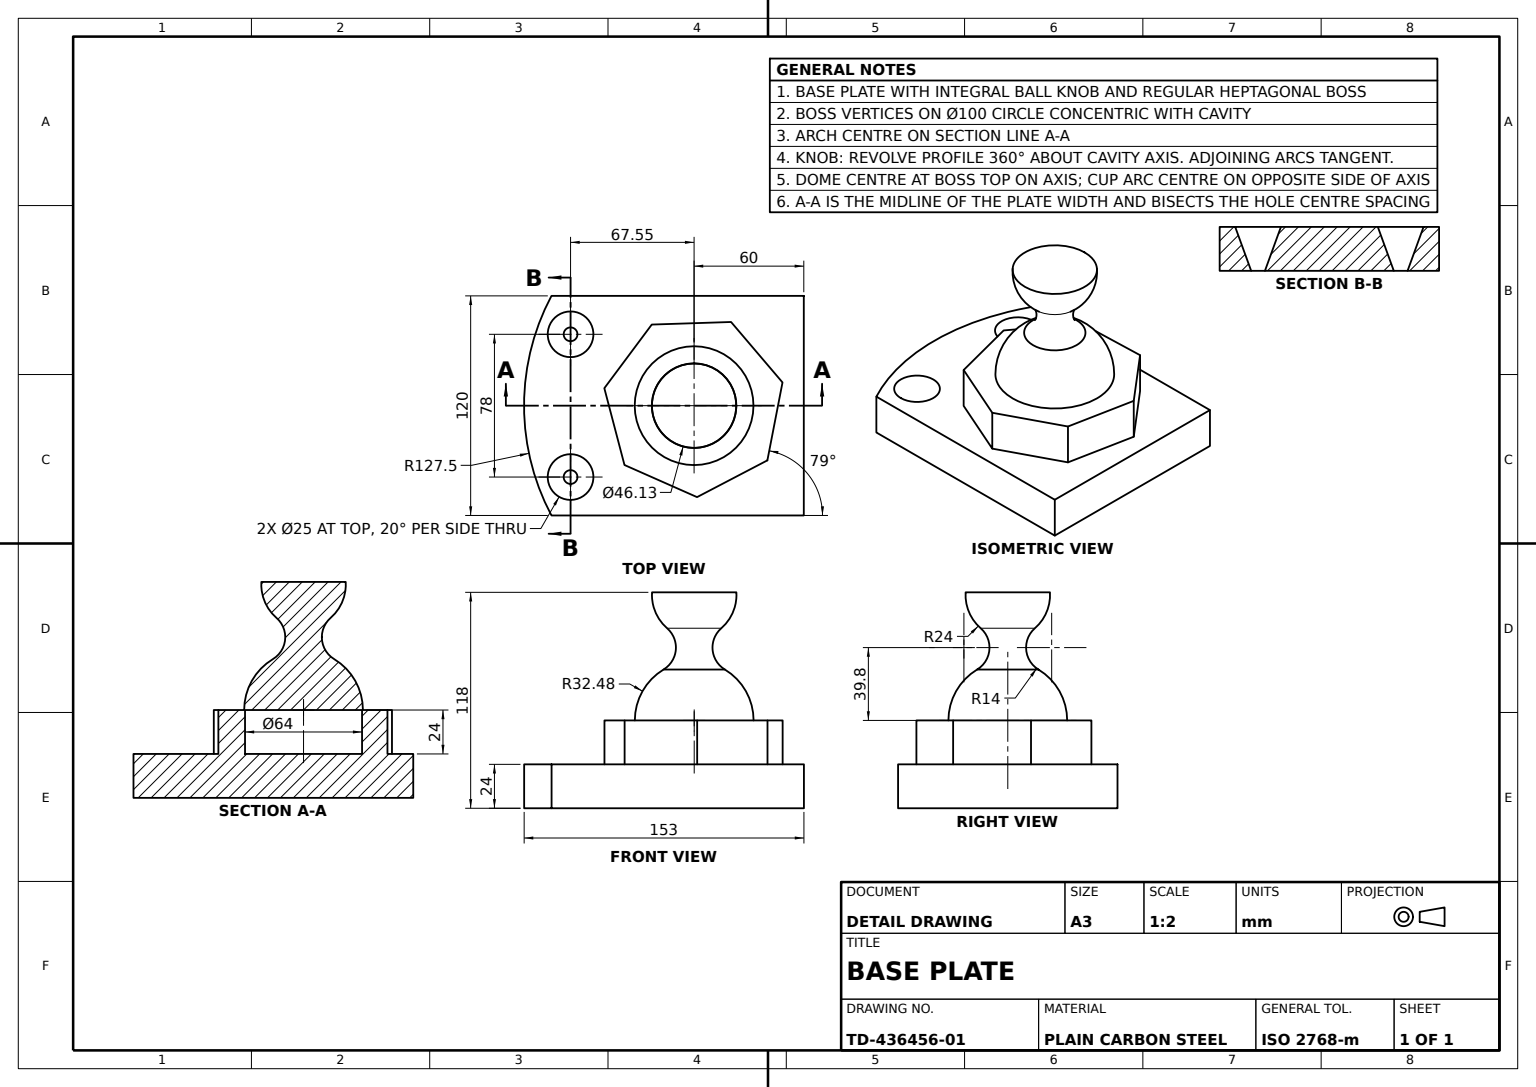
from build123d import *

# Parameters (mm, degrees)
HEX_BOSS_SKETCH_R                 = 32
HEX_BOSS_DEPTH                    = 24
BASE_PLATE_DEPTH                  = 24
PLATE_HOLES_SKETCH_R              = 12.5
PLATE_HOLES_2X_25_DEPTH           = 24
PLATE_HOLES_2X_25_DRAFT           = -20
PLATE_HOLES_2X_25_PROFILE_2_DEPTH = 24
PLATE_HOLES_2X_25_PROFILE_2_DRAFT = -20


with BuildPart() as part:
    # Knob Profile Sketch → Ball Knob (revolve)
    with BuildSketch(Plane.XY, mode=Mode.PRIVATE) as ball_knob_sk:
        with BuildLine():
            Line((0, 0), (0, 70))
            Line((0, 70), (23.065, 70))
            ThreePointArc((23.065, 70), (21.241041688, 59.227069146), (14.830368725, 50.37912389))
            ThreePointArc((14.830368725, 50.37912389), (10.051448448, 38.600871321), (16.770498027, 27.811075894))
            ThreePointArc((16.770498027, 27.811075894), (28.278508674, 15.969705495), (32.476230484, 0))
            Line((32.476230484, 0), (0, 0))
        make_face()
    revolve(ball_knob_sk.sketch.rotate(Axis((0, 0, 0), (0, 1, 0)), 90), axis=Axis((0, 0, 0), (0, 1, 0)))

    # Hex Boss Sketch → Hex Boss (add)
    with BuildSketch(Plane.XZ):
        Polygon((1.619817649, 49.97375502), (-38.061115187, 32.424551049), (-49.081251981, -9.541001202), (-23.142204959, -44.321984947), (20.223394412, -45.727610023), (48.360365309, -12.699412079), (40.080994757, 29.891702182), align=None)
        with Locations(Location((0, 0, 0), (0, 0, 270))):
            Circle(HEX_BOSS_SKETCH_R, mode=Mode.SUBTRACT)
    extrude(amount=HEX_BOSS_DEPTH)

    # Base Plate Sketch → Base Plate (add)
    with BuildSketch(Plane.XZ.offset(24)):
        with BuildLine():
            Line((-78, 60), (60, 60))
            Line((60, 60), (60, -60))
            Line((60, -60), (-78, -60))
            ThreePointArc((-78, -60), (-93, 0), (-78, 60))
        make_face()
    extrude(amount=BASE_PLATE_DEPTH)


with BuildPart() as plate_holes_2x_25_tool:
    # Plate Holes Sketch → Plate Holes 2xØ25 (with draft: the straight prism first)
    with BuildSketch(Plane(origin=(0, -24, 0), x_dir=(1, 0, 0), z_dir=(0, 1, 0))):
        with Locations((-67.55, 39)):
            Circle(PLATE_HOLES_SKETCH_R)
    extrude(amount=-PLATE_HOLES_2X_25_DEPTH)
    # Plate Holes 2xØ25: the draft: its side faces are tilted about the plane it starts from
    plate_holes_2x_25_sides = [plate_holes_2x_25_tool.faces().sort_by_distance(p)[0] for p in [
        (-80.05, -36, -39),
    ]]
    draft(plate_holes_2x_25_sides, Plane(origin=(0, -24, 0), x_dir=(1, 0, 0), z_dir=(0, 1, 0)), PLATE_HOLES_2X_25_DRAFT)


with BuildPart() as part_1:
    add(part.part)

    # Plate Holes 2xØ25: cut by plate_holes_2x_25_tool
    add(plate_holes_2x_25_tool.part, mode=Mode.SUBTRACT)


with BuildPart() as plate_holes_2x_25_profile_2_tool:
    # Plate Holes Sketch → Plate Holes 2xØ25 profile 2 (with draft: the straight prism first)
    with BuildSketch(Plane(origin=(0, -24, 0), x_dir=(1, 0, 0), z_dir=(0, 1, 0))):
        with Locations((-67.55, -39)):
            Circle(PLATE_HOLES_SKETCH_R)
    extrude(amount=-PLATE_HOLES_2X_25_PROFILE_2_DEPTH)
    # Plate Holes 2xØ25 profile 2: the draft: its side faces are tilted about the plane it starts from
    plate_holes_2x_25_profile_2_sides = [plate_holes_2x_25_profile_2_tool.faces().sort_by_distance(p)[0] for p in [
        (-80.05, -36, 39),
    ]]
    draft(plate_holes_2x_25_profile_2_sides, Plane(origin=(0, -24, 0), x_dir=(1, 0, 0), z_dir=(0, 1, 0)), PLATE_HOLES_2X_25_PROFILE_2_DRAFT)


with BuildPart() as part_2:
    add(part_1.part)

    # Plate Holes 2xØ25 profile 2: cut by plate_holes_2x_25_profile_2_tool
    add(plate_holes_2x_25_profile_2_tool.part, mode=Mode.SUBTRACT)


solid = part_2.part
